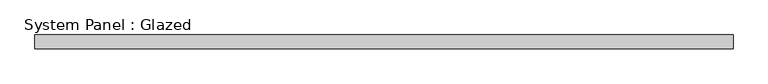
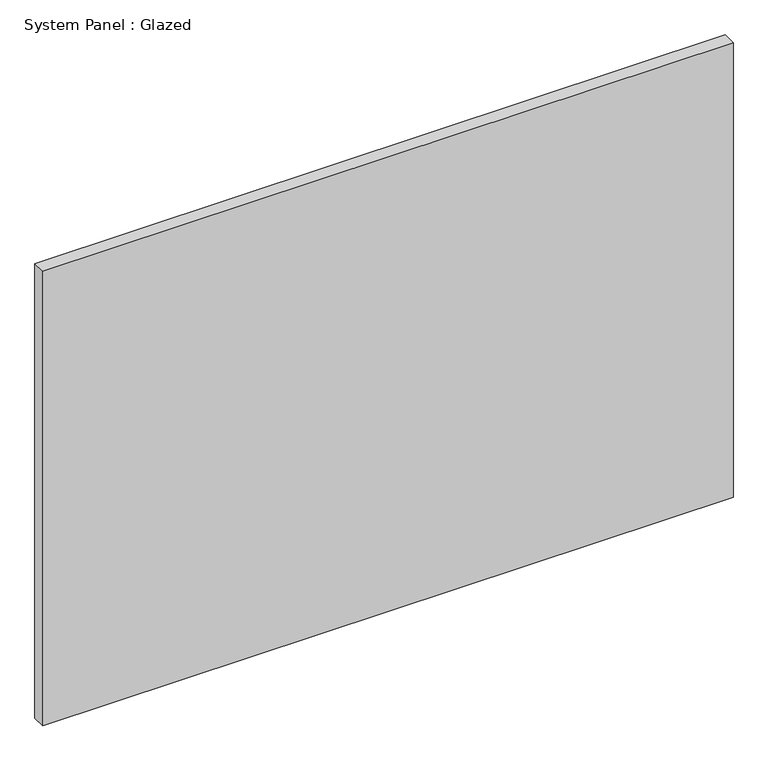
"""IFC4 building model written with IfcOpenShell, lengths in millimetres: plate geometry, System Panel : Glazed."""

from ifc_helpers import new_model, si_unit, origin, origin_with_axes, place, context, project, spatial, polyline, outline, extrude, source, transform, mapped, element, save


def system_panel_glazed_d7c040a5(model_context):
    return source(origin(), model_context, "Body", "SweptSolid", [
        extrude(outline(polyline([(649.8166667, 19.05), (-649.8166667, 19.05), (-649.8166667, 44.45), (649.8166667, 44.45), (649.8166667, 19.05)])), origin_with_axes(), (0.0, 0.0, 1.0), 904.7272807),
    ])


if __name__ == "__main__":
    model = new_model("IFC4")
    model_context = context("Model", 3, world=origin())
    ifc_project = project(units=[si_unit("LENGTHUNIT", "METRE", prefix="MILLI")], contexts=[model_context])
    site = spatial("IfcSite", under=ifc_project)
    building = spatial("IfcBuilding", under=site)
    placement = place(None, origin())
    system_panel_glazed_shape = system_panel_glazed_d7c040a5(model_context)
    element("IfcPlate", 1, ObjectType="System Panel : Glazed", at=placement, inside=building, context=model_context, shape_type="MappedRepresentation", body=[
        mapped(system_panel_glazed_shape, transform((0.0, 0.0, 0.0), x_axis=(1.0, 0.0, 0.0), y_axis=(0.0, 1.0, 0.0), z_axis=(0.0, 0.0, 1.0))),
    ])
    save(model, "model.ifc")

# Revit data of these elements
# Type "System Panel : Glazed"
#   Construction Type Id = "GSP4R"
#   Analytic Construction = "1/8 in Pilkington single glazing"
#   Visual Light Transmittance = 0.9
#   Solar Heat Gain Coefficient = 0.86
#   Heat Transfer Coefficient (U) = 1.18115 BTU/(h·ft²·°F)
#   Define Thermal Properties by = 1
# Element 1 (IfcPlate, "System Panel : Glazed")
#   Materials on its faces: "Glass"
# Materials
#   "Glass": class "Glass", colour RGB 0 128 192, transparency 0.75, Description = "Soda Lime Glass", Cost = 0
